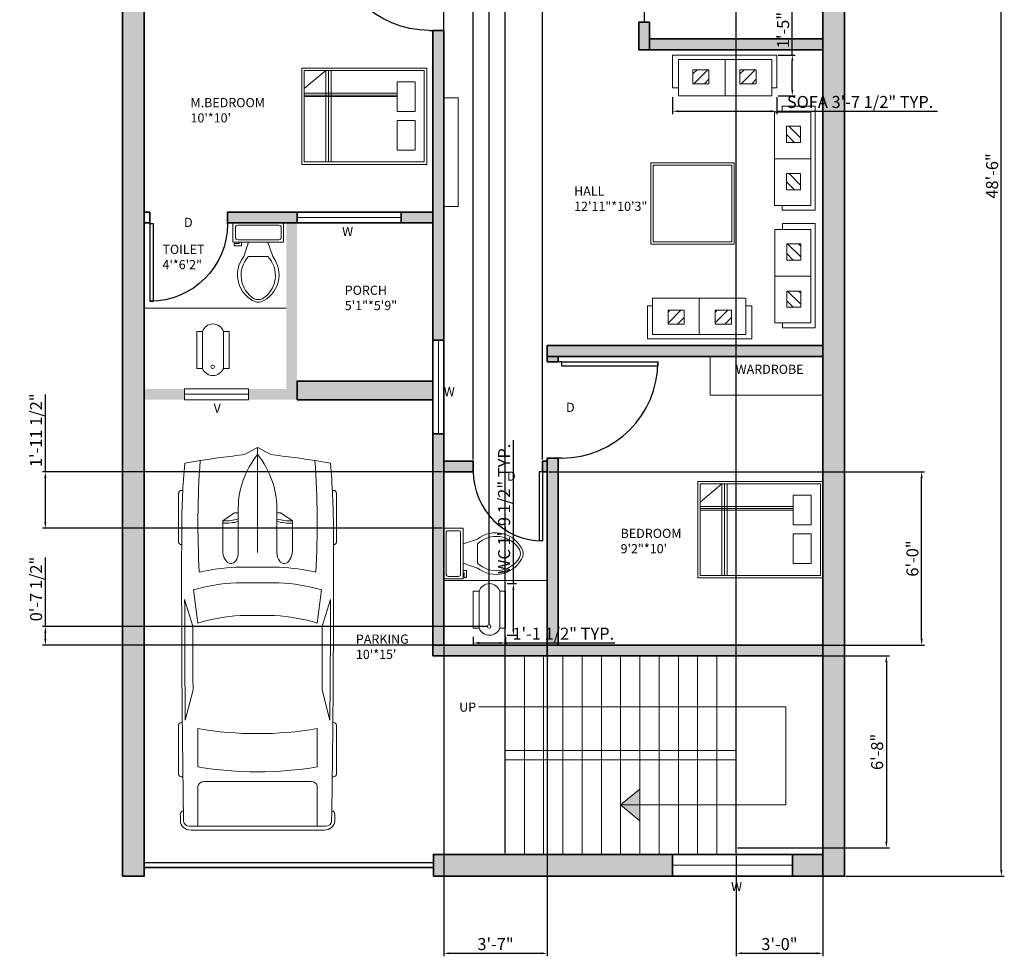
# Model space of a CAD drawing. Units: inches. Extents: x 2318 to 2727, y 1180 to 1889.
# Tile 1 of 2: x 2318 to 2727, y 1180 to 1570. Entities that reach past the tile are written whole.
import ezdxf

# ---------------------------------------------------------------- set-up
doc = ezdxf.new("R2010")
doc.units = ezdxf.units.IN
for name, color, linetype, lineweight in [('A-ANNO-DIMS', 2, 'Continuous', 18), ('A-ANNO-SYMB', 7, 'Continuous', 18), ('A-ANNO-TEXT', 7, 'Continuous', 18), ('A-AREA-IDEN', 7, 'Continuous', 18), ('A-FLOR', 7, 'Continuous', 18), ('A-FLOR-CASE', 52, 'Continuous', 20), ('A-FLOR-FIXT', 9, 'Continuous', 18), ('A-FLOR-STRS', 7, 'Continuous', 18), ('A-FURN', 52, 'Continuous', 18), ('A-WALL-PATT', 192, 'Continuous', 13), ('BED', 52, 'Continuous', 18), ('CAR', 90, 'Continuous', 13), ('DOOR', 20, 'Continuous', 25), ('WALL', 192, 'Continuous', 35), ('WIND', 130, 'Continuous', 20)]:
    doc.layers.add(name, color=color, linetype=linetype, lineweight=lineweight)
doc.styles.get("Standard").update_dxf_attribs({"font": 'arial.ttf'})
doc.dimstyles.new('ISO-25', dxfattribs={"dimtxt": 5, "dimasz": 2.5, "dimexe": 1.25, "dimexo": 0.625, "dimtad": 1, "dimdec": 0, "dimlunit": 4, "dimtxsty": 'Standard', "dimcen": 2.5, "dimadec": 0, "dimazin": 0, "dimtfac": 1, "dimtdec": 0, "dimtmove": 0, "dimatfit": 3, "dimfxl": 1, "dimarcsym": 0})

# ---------------------------------------------------------------- blocks, each defined once
blk = doc.blocks.new('*U6')
for p, q in [((46.55, 38.89), (22.35, 38.89)), ((136.7, 38.89), (160.9, 38.89)), ((21.1, 37.41), (21.1, 36.83)), ((47.8, 37.39), (47.8, 37.41)), ((87.99, 31.87), (74.76, 35.92)), ((134.31, 35.6), (119.29, 31.78)), ((135.45, 37.07), (135.45, 37.41)), ((162.15, 37.41), (162.15, 36.77)), ((70.03, 31.54), (86.41, 29.35)), ((138.42, 29.35), (157.25, 29.35)), ((186.47, 29.35), (167.01, 29.35)), ((186.47, -33.5), (186.47, 33.5)), ((188.4, -32.76), (188.4, 32.76)), ((164.52, 26.39), (164.52, -26.39)), ((32.27, 11.63), (36.13, 17.17)), ((36.13, 17.17), (50.94, 17.17)), ((32.12, 9.51), (32.12, 11.15)), ((58.92, -10.77), (58.92, 10.77)), ((66.55, -10.53), (66.55, 10.53)), ((186.47, -10.53), (186.47, 10.53)), ((3.27, 6.13), (0.1, 0.41)), ((29.77, 9.51), (51.68, 9.51)), ((82.74, 8.5), (82.74, -8.5)), ((0, 0), (51.68, 0)), ((0.1, -0.41), (3.27, -6.13)), ((29.77, -9.51), (51.68, -9.51)), ((32.12, -9.51), (32.12, -11.15)), ((32.27, -11.63), (36.13, -17.17)), ((36.13, -17.17), (50.94, -17.17)), ((86.41, -29.35), (70.03, -31.54)), ((87.99, -31.87), (74.76, -35.92)), ((134.31, -35.6), (119.29, -31.78)), ((157.25, -29.35), (138.42, -29.35)), ((167.01, -29.35), (186.47, -29.35)), ((21.1, -37.41), (21.1, -36.83)), ((47.8, -37.39), (47.8, -37.41)), ((135.45, -37.07), (135.45, -37.41)), ((162.15, -37.41), (162.15, -36.77)), ((46.55, -38.89), (22.35, -38.89)), ((136.7, -38.89), (160.9, -38.89))]:
    blk.add_line(p, q)
for centre, major_axis, ratio, start_param, end_param in [((22.35, 37.41), (0, -1.48), 0.842304, 3.141593, 4.712389), ((46.55, 37.41), (0, 1.48), 0.842304, -1.570796, 0), ((136.7, 37.41), (0, -1.48), 0.842304, 3.141593, 4.712389), ((160.9, 37.41), (0, 1.48), 0.842304, -1.570796, 0), ((266.03, -27.52), (0, 313.31), 0.842304, 1.367076, 1.39176), ((41.19, -490.86), (0, 528.23), 0.842304, 0.00281, 0.075598), ((64.48, -10555.62), (0, 10593.03), 0.842304, -0.013397, 0.002797), ((64.48, -10555.62), (0, -10591.55), 0.842304, 3.133765, 3.140441), ((180.63, 35.84), (0, 2.22), 0.842304, -0.013017, 1.249894), ((64.48, -10556.36), (0, 10595.31), 0.842304, -0.013397, -0.013017), ((183.98, 33.5), (0, -2.96), 0.842304, 1.570796, 3.128196), ((183.98, 32.76), (0, -5.25), 0.842304, 1.570796, 3.128196), ((37.47, -593.96), (0, -623.33), 0.842304, 3.096046, 3.200911), ((135.29, 5.39), (0, 81.77), 0.842304, 1.245306, 1.50788), ((149.6, 2.8), (0, -79.58), 0.842304, 4.372215, 4.640744), ((95.79, -3666.35), (0, -3698.24), 0.842304, 3.134049, 3.144098), ((17.08, 0), (0, 147.02), 0.842304, 4.511394, 4.913384), ((35.91, 0), (0, 147.02), 0.842304, 4.511394, 4.913384), ((167.01, 26.39), (0, 2.96), 0.842304, 0, 1.570796), ((259.18, -27.52), (0, -305.3), 0.842304, 4.528606, 4.561838), ((134.4, 5.39), (0, -89.78), 0.842304, 4.449482, 4.652344), ((-204.49, 52.4), (0, -250.96), 0.842304, 1.385369, 1.434372), ((13.04, 17.01), (0, 27.42), 0.842304, 4.435146, 4.718221), ((14.2, 17.01), (0, 27.42), 0.842304, 4.435146, 4.718221), ((50.79, 13.34), (6.34, -0.36), 0.603834, -1.395552, 1.581315), ((32.75, 11.15), (0, 0.74), 0.842304, 0.879714, 1.570796), ((29.77, -46.66), (0, 56.17), 0.842304, 0, 0.590319), ((0.62, 0), (0, -0.74), 0.842304, 4.131459, 5.293319), ((29.77, 46.66), (0, 56.17), 0.842304, 2.551274, 3.141593), ((-204.49, -52.4), (0, 250.96), 0.842304, -1.434372, -1.385369), ((13.04, -17.01), (0, -27.42), 0.842304, 1.564964, 1.848039), ((14.2, -17.01), (0, -27.42), 0.842304, 1.564964, 1.848039), ((149.6, -2.8), (0, -79.58), 0.842304, -1.499151, -1.230623), ((32.75, -11.15), (0, -0.74), 0.842304, 4.712389, 5.403472), ((134.4, -5.39), (0, -89.78), 0.842304, -1.510751, -1.307889), ((135.29, -5.39), (0, -81.77), 0.842304, -1.50788, -1.245306), ((259.18, 27.52), (0, 305.3), 0.842304, 1.721348, 1.754579), ((266.03, 27.52), (0, 313.31), 0.842304, 1.749832, 1.774517), ((37.47, 593.96), (0, -623.33), 0.842304, -0.059319, 0.045547), ((167.01, -26.39), (0, -2.96), 0.842304, 4.712389, 6.283185), ((95.79, 3666.35), (0, -3698.24), 0.842304, -0.002505, 0.007544), ((183.98, -33.5), (0, 2.96), 0.842304, 3.15499, 4.712389), ((183.98, -32.76), (0, -5.25), 0.842304, 0.013397, 1.570796), ((41.19, 490.86), (0, -528.23), 0.842304, -0.075598, -0.00281), ((22.35, -37.41), (0, 1.48), 0.842304, 1.570796, 3.141593), ((64.48, 10555.62), (0, 10593.03), 0.842304, 3.138796, 3.15499), ((46.55, -37.41), (0, -1.48), 0.842304, 0, 1.570796), ((64.48, 10555.62), (0, -10591.55), 0.842304, 0.001152, 0.007828), ((136.7, -37.41), (0, -1.48), 0.842304, -1.570796, 0), ((160.9, -37.41), (0, 1.48), 0.842304, 3.141593, 4.712389), ((180.63, -35.84), (0, -2.22), 0.842304, -1.249894, 0.013017), ((64.48, 10556.36), (0, 10595.31), 0.842304, 3.15461, 3.15499)]:
    blk.add_ellipse(centre, major_axis=major_axis, ratio=ratio, start_param=start_param, end_param=end_param)
at = {"extrusion": (0, 0, -1)}
blk.add_ellipse((50.79, -13.34), major_axis=(6.34, 0.36), ratio=0.603834, start_param=-1.395552, end_param=1.581315, dxfattribs=at)
blk = doc.blocks.new('*U2')
for p, q in [((0, 0), (0, -6)), ((40, 0), (40, -6))]:
    blk.add_line(p, q)
blk.add_lwpolyline([(0, 0), (0, 40), (1.75, 40), (1.75, 0)], close=True)
blk.add_arc((0, 0), 40, 0, 90)
blk = doc.blocks.new('*U4')
for p, q in [((9.5, -6), (9.5, -2)), ((-8, -8.5), (-8, -8)), ((-7, -8), (-7, -9.5)), ((-4, -8), (-6, -14)), ((4, -8), (6, -14)), ((-10, -8.5), (-8, -8.5)), ((-10, -9.5), (-10, -8.5)), ((-7, -9.5), (-10, -9.5)), ((4, -14), (-4, -14))]:
    blk.add_line(p, q)
blk.add_lwpolyline([(10.5, -8), (10.5, 0), (-10.5, 0), (-10.5, -8)], close=True)
for points in [[(-9.5, -2), (-9.5, -6)], [(8.5, -1), (-8.5, -1)], [(-8.5, -7), (8.5, -7)]]:
    blk.add_lwpolyline(points)
for centre, radius, start, end in [((-8.62, -1.88), 0.884, 81.8699, 188.1301), ((8.62, -1.88), 0.884, 351.8699, 98.1301), ((-8.62, -6.12), 0.884, 171.8699, 278.1301), ((8.62, -6.12), 0.884, 261.8699, 8.1301), ((3.52, -21.58), 12.17, 141.4691, 247.9714), ((4.2, -21.82), 11.33, 136.3677, 238.9468), ((-3.52, -21.58), 12.17, 292.0284, 38.5307), ((-4.2, -21.82), 11.33, 301.053, 43.6321), ((0, -27.88), 4, 245.7318, 294.2682), ((0, -29), 4, 254.8605, 285.1395)]:
    blk.add_arc(centre, radius, start, end)
blk = doc.blocks.new('*D9')
at = {"layer": 'A-ANNO-DIMS', "color": 0, "lineweight": -2, "transparency": 16777216}
for p, q in [((2616.06, 1305.12), (2679.12, 1305.12)), ((2677.87, 1302.62), (2677.87, 1227.86)), ((2616.06, 1225.36), (2679.12, 1225.36))]:
    blk.add_line(p, q, dxfattribs=at)
at = {"layer": 'A-ANNO-DIMS', "color": 0, "transparency": 16777216}
for points in [[(2677.45, 1302.62), (2678.29, 1302.62), (2677.87, 1305.12)], [(2677.45, 1227.86), (2678.29, 1227.86), (2677.87, 1225.36)]]:
    blk.add_solid(points, dxfattribs=at)
at = {"layer": 'Defpoints', "color": 0, "transparency": 16777216}
for p in [(2615.43, 1305.12), (2615.43, 1225.36), (2677.87, 1225.36)]:
    blk.add_point(p, dxfattribs=at)
at = {"layer": 'A-ANNO-DIMS', "color": 0, "transparency": 16777216, "insert": (2674.69, 1265.24), "char_height": 5, "attachment_point": 5, "rotation": 90}
blk.add_mtext('6\'-8"', dxfattribs=at)
blk = doc.blocks.new('*D10')
at = {"layer": 'A-ANNO-DIMS', "color": 0, "lineweight": -2, "transparency": 16777216}
for p, q in [((2661.06, 1795.62), (2726.9, 1795.62)), ((2725.65, 1216.12), (2725.65, 1793.12)), ((2661.06, 1213.62), (2726.9, 1213.62))]:
    blk.add_line(p, q, dxfattribs=at)
at = {"layer": 'A-ANNO-DIMS', "color": 0, "transparency": 16777216}
for points in [[(2725.23, 1793.12), (2726.06, 1793.12), (2725.65, 1795.62)], [(2725.23, 1216.12), (2726.06, 1216.12), (2725.65, 1213.62)]]:
    blk.add_solid(points, dxfattribs=at)
at = {"layer": 'Defpoints', "color": 0, "transparency": 16777216}
for p in [(2660.43, 1795.62), (2725.65, 1795.62), (2660.43, 1213.62)]:
    blk.add_point(p, dxfattribs=at)
at = {"layer": 'A-ANNO-DIMS', "color": 0, "transparency": 16777216, "insert": (2722.47, 1504.62), "char_height": 5, "attachment_point": 5, "rotation": 90}
blk.add_mtext('48\'-6"', dxfattribs=at)
blk = doc.blocks.new('BED-DOUBLE')
for p, q in [((1, 31.46), (10.01, 39.03)), ((10.01, 39.03), (10.01, 1)), ((11.11, 39.03), (11.11, 1)), ((12.24, 39.03), (12.24, 1)), ((39.72, 29.6), (1, 29.6)), ((1, 28.8), (39.72, 28.8)), ((39.72, 28.17), (1, 28.17))]:
    blk.add_line(p, q)
for points in [[(51.96, 40.03), (0, 40.03), (0, 0), (51.96, 0)], [(50.96, 39.03), (1, 39.03), (1, 1), (50.96, 1)], [(47.18, 34.34), (39.72, 34.34), (39.72, 22.01), (47.18, 22.01)], [(47.18, 18.28), (39.72, 18.28), (39.72, 5.95), (47.18, 5.95)]]:
    blk.add_lwpolyline(points, close=True)
blk = doc.blocks.new('WC-SQUAT')
for points in [[(0, 2.9), (2.39, 2.9), (2.39, 18.34), (0, 18.34)], [(11.06, 2.9), (13.46, 2.9), (13.46, 18.34), (11.06, 18.34)]]:
    blk.add_lwpolyline(points, close=True)
for points in [[(2.39, 18.28), (2.39, 2.9)], [(11.06, 2.9), (11.06, 18.28)]]:
    blk.add_lwpolyline(points)
blk.add_circle((6.6, 3.6), 0.726)
for centre, radius, start, end in [((6.73, 16.89), 4.55, 17.8162, 162.1838), ((6.73, 4.69), 4.69, 202.5147, 337.4853)]:
    blk.add_arc(centre, radius, start, end)
blk = doc.blocks.new('SOFA-TWO-SEAT')
h = blk.add_hatch()
h.set_pattern_fill('ANSI31', color=256)
h.set_pattern_definition([(45, (-2589.011, -1538.005), (-2.245064, 2.245064), [])])
h.paths.add_polyline_path([(15.14, 10.8), (8.38, 10.8), (8.38, 4.98), (15.14, 4.98)])
h = blk.add_hatch()
h.set_pattern_fill('ANSI31', color=256)
h.set_pattern_definition([(45, (-2569.365, -1538.005), (-2.245064, 2.245064), [])])
h.paths.add_polyline_path([(34.79, 10.8), (28.03, 10.8), (28.03, 4.98), (34.79, 4.98)])
for p, q in [((0, 3.19), (0, 16.86)), ((0, 16.86), (43.28, 16.86)), ((43.28, 16.86), (43.28, 3.19)), ((21.85, 0), (21.85, 15.05)), ((2.44, 3.19), (0, 3.19)), ((43.28, 3.19), (41.27, 3.19))]:
    blk.add_line(p, q)
for points in [[(2.44, 0), (41.27, 0), (41.27, 15.05), (2.44, 15.05)], [(8.38, 4.98), (15.14, 4.98), (15.14, 10.8), (8.38, 10.8)], [(28.03, 4.98), (34.79, 4.98), (34.79, 10.8), (28.03, 10.8)]]:
    blk.add_lwpolyline(points, close=True)
blk = doc.blocks.new('*D16')
at = {"layer": 'A-ANNO-DIMS', "color": 0, "lineweight": -2, "transparency": 16777216}
for p, q in [((2589.01, 1537.38), (2589.01, 1530.26)), ((2632.29, 1537.38), (2632.29, 1530.26)), ((2591.51, 1531.51), (2629.79, 1531.51)), ((2632.29, 1531.51), (2699.11, 1531.51))]:
    blk.add_line(p, q, dxfattribs=at)
at = {"layer": 'A-ANNO-DIMS', "color": 0, "transparency": 16777216}
for points in [[(2591.51, 1531.93), (2591.51, 1531.1), (2589.01, 1531.51)], [(2629.79, 1531.93), (2629.79, 1531.1), (2632.29, 1531.51)]]:
    blk.add_solid(points, dxfattribs=at)
at = {"layer": 'Defpoints', "color": 0, "transparency": 16777216}
for p in [(2589.01, 1538), (2632.29, 1538), (2632.29, 1531.51)]:
    blk.add_point(p, dxfattribs=at)
at = {"layer": 'A-ANNO-DIMS', "color": 0, "transparency": 16777216, "insert": (2666.95, 1534.73), "char_height": 5, "attachment_point": 5}
blk.add_mtext('SOFA 3\'-7 1/2" TYP.', dxfattribs=at)
blk = doc.blocks.new('*D17')
at = {"layer": 'A-ANNO-DIMS', "color": 0, "lineweight": -2, "transparency": 16777216}
for p, q in [((2638.78, 1554.87), (2638.78, 1588.62)), ((2632.92, 1554.87), (2640.03, 1554.87)), ((2638.78, 1540.5), (2638.78, 1552.37)), ((2632.92, 1538), (2640.03, 1538))]:
    blk.add_line(p, q, dxfattribs=at)
at = {"layer": 'A-ANNO-DIMS', "color": 0, "transparency": 16777216}
for points in [[(2638.37, 1552.37), (2639.2, 1552.37), (2638.78, 1554.87)], [(2638.37, 1540.5), (2639.2, 1540.5), (2638.78, 1538)]]:
    blk.add_solid(points, dxfattribs=at)
at = {"layer": 'Defpoints', "color": 0, "transparency": 16777216}
for p in [(2632.29, 1554.87), (2638.78, 1554.87), (2632.29, 1538)]:
    blk.add_point(p, dxfattribs=at)
at = {"layer": 'A-ANNO-DIMS', "color": 0, "transparency": 16777216, "insert": (2635.61, 1572.99), "char_height": 5, "attachment_point": 5, "rotation": 90}
blk.add_mtext('1\'-5" TYP.', dxfattribs=at)
blk = doc.blocks.new('*D20')
at = {"layer": 'A-ANNO-DIMS', "color": 0, "lineweight": -2, "transparency": 16777216}
for p, q in [((2522.86, 1335.18), (2522.86, 1394.84)), ((2520.26, 1335.18), (2524.11, 1335.18)), ((2522.86, 1316.23), (2522.86, 1332.68)), ((2520.26, 1313.73), (2524.11, 1313.73))]:
    blk.add_line(p, q, dxfattribs=at)
at = {"layer": 'A-ANNO-DIMS', "color": 0, "transparency": 16777216}
for points in [[(2522.44, 1332.68), (2523.27, 1332.68), (2522.86, 1335.18)], [(2522.44, 1316.23), (2523.27, 1316.23), (2522.86, 1313.73)]]:
    blk.add_solid(points, dxfattribs=at)
at = {"layer": 'Defpoints', "color": 0, "transparency": 16777216}
for p in [(2519.64, 1335.18), (2522.86, 1335.18), (2519.64, 1313.73)]:
    blk.add_point(p, dxfattribs=at)
at = {"layer": 'A-ANNO-DIMS', "color": 0, "transparency": 16777216, "insert": (2519.65, 1366.26), "char_height": 5, "attachment_point": 5, "rotation": 90}
blk.add_mtext('WC 1\'-9 1/2" TYP.', dxfattribs=at)
blk = doc.blocks.new('*D21')
at = {"layer": 'A-ANNO-DIMS', "color": 0, "lineweight": -2, "transparency": 16777216}
for p, q in [((2506.18, 1313.11), (2506.18, 1309.26)), ((2508.68, 1310.51), (2517.14, 1310.51)), ((2519.64, 1313.11), (2519.64, 1309.26)), ((2519.64, 1310.51), (2565.05, 1310.51))]:
    blk.add_line(p, q, dxfattribs=at)
at = {"layer": 'A-ANNO-DIMS', "color": 0, "transparency": 16777216}
for points in [[(2508.68, 1310.93), (2508.68, 1310.1), (2506.18, 1310.51)], [(2517.14, 1310.93), (2517.14, 1310.1), (2519.64, 1310.51)]]:
    blk.add_solid(points, dxfattribs=at)
at = {"layer": 'Defpoints', "color": 0, "transparency": 16777216}
for p in [(2506.18, 1313.73), (2519.64, 1313.73), (2519.64, 1310.51)]:
    blk.add_point(p, dxfattribs=at)
at = {"layer": 'A-ANNO-DIMS', "color": 0, "transparency": 16777216, "insert": (2543.59, 1313.72), "char_height": 5, "attachment_point": 5}
blk.add_mtext('1\'-1 1/2" TYP.', dxfattribs=at)
blk = doc.blocks.new('*D24')
at = {"layer": 'A-ANNO-DIMS', "color": 0, "lineweight": -2, "transparency": 16777216}
for p, q in [((2519.43, 1223.25), (2519.43, 1879.97)), ((2521.93, 1878.72), (2612.93, 1878.72)), ((2615.43, 1223.25), (2615.43, 1879.97))]:
    blk.add_line(p, q, dxfattribs=at)
at = {"layer": 'A-ANNO-DIMS', "color": 0, "transparency": 16777216}
for points in [[(2521.93, 1879.14), (2521.93, 1878.3), (2519.43, 1878.72)], [(2612.93, 1879.14), (2612.93, 1878.3), (2615.43, 1878.72)]]:
    blk.add_solid(points, dxfattribs=at)
at = {"layer": 'Defpoints', "color": 0, "transparency": 16777216}
for p in [(2615.43, 1878.72), (2519.43, 1222.62), (2615.43, 1222.62)]:
    blk.add_point(p, dxfattribs=at)
at = {"layer": 'A-ANNO-DIMS', "color": 0, "transparency": 16777216, "insert": (2567.43, 1881.9), "char_height": 5, "attachment_point": 5}
blk.add_mtext('8\'-0"', dxfattribs=at)
blk = doc.blocks.new('*D25')
at = {"layer": 'A-ANNO-DIMS', "color": 0, "lineweight": -2, "transparency": 16777216}
for p, q in [((2615.43, 1222), (2615.43, 1180.27)), ((2651.43, 1222), (2651.43, 1180.27)), ((2617.93, 1181.52), (2648.93, 1181.52))]:
    blk.add_line(p, q, dxfattribs=at)
at = {"layer": 'A-ANNO-DIMS', "color": 0, "transparency": 16777216}
for points in [[(2617.93, 1181.94), (2617.93, 1181.1), (2615.43, 1181.52)], [(2648.93, 1181.94), (2648.93, 1181.1), (2651.43, 1181.52)]]:
    blk.add_solid(points, dxfattribs=at)
at = {"layer": 'Defpoints', "color": 0, "transparency": 16777216}
for p in [(2615.43, 1222.62), (2651.43, 1222.62), (2651.43, 1181.52)]:
    blk.add_point(p, dxfattribs=at)
at = {"layer": 'A-ANNO-DIMS', "color": 0, "transparency": 16777216, "insert": (2633.43, 1184.7), "char_height": 5, "attachment_point": 5}
blk.add_mtext('3\'-0"', dxfattribs=at)
blk = doc.blocks.new('*D26')
at = {"layer": 'A-ANNO-DIMS', "color": 0, "lineweight": -2, "transparency": 16777216}
for p, q in [((2493.93, 1309), (2493.93, 1180.27)), ((2536.93, 1309), (2536.93, 1180.27)), ((2496.43, 1181.52), (2534.43, 1181.52))]:
    blk.add_line(p, q, dxfattribs=at)
at = {"layer": 'A-ANNO-DIMS', "color": 0, "transparency": 16777216}
for points in [[(2496.43, 1181.94), (2496.43, 1181.1), (2493.93, 1181.52)], [(2534.43, 1181.94), (2534.43, 1181.1), (2536.93, 1181.52)]]:
    blk.add_solid(points, dxfattribs=at)
at = {"layer": 'Defpoints', "color": 0, "transparency": 16777216}
for p in [(2493.93, 1309.62), (2536.93, 1309.62), (2536.93, 1181.52)]:
    blk.add_point(p, dxfattribs=at)
at = {"layer": 'A-ANNO-DIMS', "color": 0, "transparency": 16777216, "insert": (2515.43, 1184.7), "char_height": 5, "attachment_point": 5}
blk.add_mtext('3\'-7"', dxfattribs=at)
blk = doc.blocks.new('*D27')
at = {"layer": 'A-ANNO-DIMS', "color": 0, "lineweight": -2, "transparency": 16777216}
for p, q in [((2537.56, 1381.62), (2693.78, 1381.62)), ((2692.53, 1312.12), (2692.53, 1379.12)), ((2537.56, 1309.62), (2693.78, 1309.62))]:
    blk.add_line(p, q, dxfattribs=at)
at = {"layer": 'A-ANNO-DIMS', "color": 0, "transparency": 16777216}
for points in [[(2692.12, 1379.12), (2692.95, 1379.12), (2692.53, 1381.62)], [(2692.12, 1312.12), (2692.95, 1312.12), (2692.53, 1309.62)]]:
    blk.add_solid(points, dxfattribs=at)
at = {"layer": 'Defpoints', "color": 0, "transparency": 16777216}
for p in [(2536.93, 1381.62), (2692.53, 1381.62), (2536.93, 1309.62)]:
    blk.add_point(p, dxfattribs=at)
at = {"layer": 'A-ANNO-DIMS', "color": 0, "transparency": 16777216, "insert": (2689.36, 1345.62), "char_height": 5, "attachment_point": 5, "rotation": 90}
blk.add_mtext('6\'-0"', dxfattribs=at)
blk = doc.blocks.new('*D28')
at = {"layer": 'A-ANNO-DIMS', "color": 0, "lineweight": -2, "transparency": 16777216}
for p, q in [((2506.2, 1386.75), (2506.2, 1879.97)), ((2508.7, 1878.72), (2532.52, 1878.72)), ((2535.02, 1386.75), (2535.02, 1879.97))]:
    blk.add_line(p, q, dxfattribs=at)
at = {"layer": 'A-ANNO-DIMS', "color": 0, "transparency": 16777216}
for points in [[(2508.7, 1879.14), (2508.7, 1878.3), (2506.2, 1878.72)], [(2532.52, 1879.14), (2532.52, 1878.3), (2535.02, 1878.72)]]:
    blk.add_solid(points, dxfattribs=at)
at = {"layer": 'Defpoints', "color": 0, "transparency": 16777216}
for p in [(2535.02, 1878.72), (2506.2, 1386.12), (2535.02, 1386.12)]:
    blk.add_point(p, dxfattribs=at)
at = {"layer": 'A-ANNO-DIMS', "color": 0, "transparency": 16777216, "insert": (2520.61, 1881.9), "char_height": 5, "attachment_point": 5}
blk.add_mtext('2\'-5"', dxfattribs=at)
blk = doc.blocks.new('*D29')
at = {"layer": 'A-ANNO-DIMS', "color": 0, "lineweight": -2, "transparency": 16777216}
for p, q in [((2493.93, 1386.75), (2493.93, 1879.97)), ((2496.43, 1878.72), (2503.7, 1878.72)), ((2506.2, 1386.75), (2506.2, 1879.97)), ((2506.2, 1878.72), (2534.42, 1878.72))]:
    blk.add_line(p, q, dxfattribs=at)
at = {"layer": 'A-ANNO-DIMS', "color": 0, "transparency": 16777216}
for points in [[(2496.43, 1879.14), (2496.43, 1878.3), (2493.93, 1878.72)], [(2503.7, 1879.14), (2503.7, 1878.3), (2506.2, 1878.72)]]:
    blk.add_solid(points, dxfattribs=at)
at = {"layer": 'Defpoints', "color": 0, "transparency": 16777216}
for p in [(2506.2, 1878.72), (2493.93, 1386.12), (2506.2, 1386.12)]:
    blk.add_point(p, dxfattribs=at)
at = {"layer": 'A-ANNO-DIMS', "color": 0, "transparency": 16777216, "insert": (2521.56, 1881.93), "char_height": 5, "attachment_point": 5}
blk.add_mtext('1\'-0 1/2"', dxfattribs=at)
blk = doc.blocks.new('*D30')
at = {"layer": 'A-ANNO-DIMS', "color": 0, "lineweight": -2, "transparency": 16777216}
for p, q in [((2493.93, 1310.25), (2493.93, 1879.97)), ((2496.43, 1878.72), (2510.28, 1878.72)), ((2512.78, 1317.96), (2512.78, 1879.97))]:
    blk.add_line(p, q, dxfattribs=at)
at = {"layer": 'A-ANNO-DIMS', "color": 0, "transparency": 16777216}
for points in [[(2496.43, 1879.14), (2496.43, 1878.3), (2493.93, 1878.72)], [(2510.28, 1879.14), (2510.28, 1878.3), (2512.78, 1878.72)]]:
    blk.add_solid(points, dxfattribs=at)
at = {"layer": 'Defpoints', "color": 0, "transparency": 16777216}
for p in [(2512.78, 1878.72), (2512.78, 1317.33), (2493.93, 1309.62)]:
    blk.add_point(p, dxfattribs=at)
at = {"layer": 'A-ANNO-DIMS', "color": 0, "transparency": 16777216, "insert": (2503.36, 1881.86), "char_height": 5, "attachment_point": 5}
blk.add_mtext('1\'-7"', dxfattribs=at)
blk = doc.blocks.new('*D31')
at = {"layer": 'A-ANNO-DIMS', "color": 0, "lineweight": -2, "transparency": 16777216}
for p, q in [((2328.33, 1317.33), (2328.33, 1346.02)), ((2512.16, 1317.33), (2327.08, 1317.33)), ((2328.33, 1312.12), (2328.33, 1314.83)), ((2493.31, 1309.62), (2327.08, 1309.62))]:
    blk.add_line(p, q, dxfattribs=at)
at = {"layer": 'A-ANNO-DIMS', "color": 0, "transparency": 16777216}
for points in [[(2327.92, 1314.83), (2328.75, 1314.83), (2328.33, 1317.33)], [(2327.92, 1312.12), (2328.75, 1312.12), (2328.33, 1309.62)]]:
    blk.add_solid(points, dxfattribs=at)
at = {"layer": 'Defpoints', "color": 0, "transparency": 16777216}
for p in [(2328.33, 1317.33), (2512.78, 1317.33), (2493.93, 1309.62)]:
    blk.add_point(p, dxfattribs=at)
at = {"layer": 'A-ANNO-DIMS', "color": 0, "transparency": 16777216, "insert": (2325.12, 1332.93), "char_height": 5, "attachment_point": 5, "rotation": 90}
blk.add_mtext('0\'-7 1/2"', dxfattribs=at)
blk = doc.blocks.new('*D32')
at = {"layer": 'A-ANNO-DIMS', "color": 0, "lineweight": -2, "transparency": 16777216}
for p, q in [((2328.33, 1381.62), (2328.33, 1413.73)), ((2493.31, 1381.62), (2327.08, 1381.62)), ((2328.33, 1360.67), (2328.33, 1379.12)), ((2493.31, 1358.17), (2327.08, 1358.17))]:
    blk.add_line(p, q, dxfattribs=at)
at = {"layer": 'A-ANNO-DIMS', "color": 0, "transparency": 16777216}
for points in [[(2327.92, 1379.12), (2328.75, 1379.12), (2328.33, 1381.62)], [(2327.92, 1360.67), (2328.75, 1360.67), (2328.33, 1358.17)]]:
    blk.add_solid(points, dxfattribs=at)
at = {"layer": 'Defpoints', "color": 0, "transparency": 16777216}
for p in [(2328.33, 1381.62), (2493.93, 1381.62), (2493.93, 1358.17)]:
    blk.add_point(p, dxfattribs=at)
at = {"layer": 'A-ANNO-DIMS', "color": 0, "transparency": 16777216, "insert": (2325.12, 1398.92), "char_height": 5, "attachment_point": 5, "rotation": 90}
blk.add_mtext('1\'-11 1/2"', dxfattribs=at)

msp = doc.modelspace()

# ---------------------------------------------------------------- hatches: boundary and pattern name
at = {"layer": 'A-ANNO-SYMB'}
h = msp.add_hatch(color=256, dxfattribs=at)
h.dxf.hatch_style = 1
h.paths.add_polyline_path([(2575.43, 1249.74), (2567.43, 1243.17), (2575.43, 1243.17)])
h.paths.add_polyline_path([(2575.43, 1243.17), (2567.43, 1243.17), (2575.43, 1236.61)])
at = {"layer": 'A-WALL-PATT'}
h = msp.add_hatch(color=256, dxfattribs=at)
h.dxf.hatch_style = 1
h.paths.add_polyline_path([(2651.43, 1795.62), (2360.43, 1795.62), (2360.43, 1786.62), (2369.43, 1786.62), (2651.43, 1786.62)])
h.paths.add_polyline_path([(2481.93, 1786.62), (2477.43, 1786.62), (2477.43, 1778.41), (2481.93, 1778.41)])
h.paths.add_polyline_path([(2481.93, 1750.36), (2477.43, 1750.36), (2477.43, 1738.62), (2481.93, 1738.62)])
h.paths.add_polyline_path([(2369.43, 1786.62), (2360.43, 1786.62), (2360.43, 1213.62), (2369.43, 1213.62)])
h.paths.add_polyline_path([(2660.43, 1795.62), (2651.43, 1795.62), (2651.43, 1786.62), (2651.43, 1213.62), (2660.43, 1213.62)])
h.paths.add_polyline_path([(2496.41, 1614.12), (2369.43, 1614.12), (2369.43, 1609.62), (2496.41, 1609.62)])
h.paths.add_polyline_path([(2651.43, 1614.12), (2570.03, 1614.12), (2570.03, 1609.62), (2651.43, 1609.62)])
h.paths.add_polyline_path([(2579.43, 1609.62), (2574.93, 1609.62), (2574.93, 1602.98), (2579.43, 1602.98)])
h.paths.add_polyline_path([(2579.43, 1568.54), (2574.93, 1568.54), (2574.93, 1557.12), (2579.43, 1557.12)])
h.paths.add_polyline_path([(2651.43, 1561.62), (2579.43, 1561.62), (2579.43, 1557.12), (2651.43, 1557.12)])
h.paths.add_polyline_path([(2493.93, 1565.11), (2489.43, 1565.11), (2489.43, 1436.36), (2493.93, 1436.36)])
h.paths.add_polyline_path([(2489.43, 1419.4), (2432.93, 1419.4), (2432.93, 1411.62), (2489.43, 1411.62)])
h.paths.add_polyline_path([(2493.93, 1397.39), (2489.43, 1397.39), (2489.43, 1309.62), (2493.93, 1309.62)])
h.paths.add_polyline_path([(2506.2, 1386.12), (2493.93, 1386.12), (2493.93, 1381.62), (2506.2, 1381.62)])
h.paths.add_polyline_path([(2651.43, 1434.12), (2536.93, 1434.12), (2536.93, 1429.62), (2651.43, 1429.62)])
h.paths.add_polyline_path([(2541.43, 1429.62), (2536.93, 1429.62), (2536.93, 1427.36), (2541.43, 1427.36)])
h.paths.add_polyline_path([(2541.43, 1387.36), (2536.93, 1387.36), (2536.93, 1309.62), (2541.43, 1309.62)])
h.paths.add_polyline_path([(2536.93, 1386.12), (2535.02, 1386.12), (2535.02, 1381.8), (2535.02, 1381.62), (2536.93, 1381.62)])
h.paths.add_polyline_path([(2536.93, 1309.62), (2489.43, 1309.62), (2489.43, 1305.12), (2536.93, 1305.12)])
h.paths.add_polyline_path([(2651.43, 1309.62), (2536.93, 1309.62), (2536.93, 1305.12), (2651.43, 1305.12)])
h.paths.add_polyline_path([(2651.43, 1222.62), (2638.9, 1222.62), (2638.9, 1213.62), (2651.43, 1213.62)])
h.paths.add_polyline_path([(2588.94, 1222.62), (2489.59, 1222.62), (2489.59, 1213.62), (2588.94, 1213.62)])
h = msp.add_hatch(color=256, dxfattribs=at)
h.dxf.hatch_style = 1
h.paths.add_polyline_path([(2481.93, 1738.62), (2477.43, 1738.62), (2404.9, 1738.62), (2404.9, 1734.12), (2481.93, 1734.12)])
h.paths.add_polyline_path([(2537.33, 1738.62), (2529.86, 1738.62), (2529.86, 1734.12), (2530.43, 1734.12), (2530.43, 1614.12), (2534.93, 1614.12), (2534.93, 1734.12), (2537.33, 1734.12)])
h.paths.add_polyline_path([(2599, 1738.62), (2588.85, 1738.62), (2588.85, 1734.12), (2599, 1734.12)])
h.paths.add_polyline_path([(2651.43, 1738.62), (2645.81, 1738.62), (2645.81, 1734.12), (2651.43, 1734.12)])
h.paths.add_polyline_path([(2534.93, 1614.12), (2530.43, 1614.12), (2530.3, 1614.12), (2530.3, 1609.62), (2534.93, 1609.62)])
h.paths.add_polyline_path([(2493.93, 1609.62), (2489.43, 1609.62), (2489.43, 1605.11), (2493.93, 1605.11)])
h.paths.add_polyline_path([(2386.22, 1416.12), (2369.43, 1416.12), (2369.43, 1411.62), (2386.22, 1411.62)])
h.paths.add_polyline_path([(2432.93, 1416.12), (2432.93, 1485.12), (2428.43, 1485.12), (2428.43, 1416.12), (2412.83, 1416.12), (2412.83, 1411.62), (2428.43, 1411.62), (2432.93, 1411.62)])
h = msp.add_hatch(color=256, dxfattribs=at)
h.dxf.hatch_style = 1
h.paths.add_polyline_path([(2489.43, 1489.62), (2476.24, 1489.62), (2476.24, 1485.12), (2489.43, 1485.12)])
h.paths.add_polyline_path([(2432.93, 1489.62), (2404.06, 1489.62), (2404.06, 1485.12), (2432.93, 1485.12)])

# ---------------------------------------------------------------- linework, layer by layer
at = {"layer": 'A-ANNO-SYMB'}
for p, q in [((2508.53, 1283.98), (2636.15, 1283.98)), ((2636.15, 1283.98), (2636.15, 1243.17)), ((2567.43, 1243.17), (2575.43, 1249.74)), ((2636.15, 1243.17), (2567.43, 1243.17)), ((2567.43, 1243.17), (2575.43, 1236.61))]:
    msp.add_line(p, q, dxfattribs=at)
at = {"layer": 'A-FLOR'}
for p, q in [((2369.43, 1449.69), (2428.43, 1449.69)), ((2493.93, 1336.53), (2536.93, 1336.53))]:
    msp.add_line(p, q, dxfattribs=at)
at = {"layer": 'A-FLOR-CASE'}
for points in [[(2493.93, 1491.99), (2499.84, 1491.99), (2499.84, 1537.16), (2493.93, 1537.16)], [(2651.43, 1429.62), (2604.68, 1429.62), (2604.68, 1413.49), (2651.43, 1413.49)]]:
    msp.add_lwpolyline(points, close=True, dxfattribs=at)
at = {"layer": 'A-FLOR-STRS'}
for p, q in [((2519.43, 1305.12), (2519.43, 1222.62)), ((2527.43, 1305.12), (2527.43, 1222.62)), ((2535.43, 1305.12), (2535.43, 1222.62)), ((2543.43, 1305.12), (2543.43, 1222.62)), ((2543.43, 1305.12), (2543.43, 1222.62)), ((2551.43, 1305.12), (2551.43, 1222.62)), ((2559.43, 1305.12), (2559.43, 1222.62)), ((2567.43, 1305.12), (2567.43, 1222.62)), ((2575.43, 1305.12), (2575.43, 1222.62)), ((2583.43, 1305.12), (2583.43, 1222.62)), ((2591.43, 1305.12), (2591.43, 1222.62)), ((2599.43, 1305.12), (2599.43, 1222.62)), ((2607.43, 1305.12), (2607.43, 1222.62)), ((2651.43, 1305.12), (2615.43, 1305.12)), ((2615.43, 1305.12), (2615.43, 1222.62)), ((2615.43, 1265.87), (2519.1, 1265.87)), ((2615.43, 1261.87), (2519.1, 1261.87))]:
    msp.add_line(p, q, dxfattribs=at)
at = {"layer": 'A-FURN'}
for points in [[(2614.67, 1476.3), (2580.01, 1476.3), (2580.01, 1510.09), (2614.67, 1510.09)], [(2613.67, 1477.3), (2581.01, 1477.3), (2581.01, 1509.09), (2613.67, 1509.09)]]:
    msp.add_lwpolyline(points, close=True, dxfattribs=at)
at = {"layer": 'DOOR'}
for p, q in [((2577.18, 1602.98), (2577.18, 1568.54)), ((2489.37, 1217.14), (2369.22, 1217.14)), ((2489.59, 1219.12), (2369.43, 1219.12))]:
    msp.add_line(p, q, dxfattribs=at)
msp.add_lwpolyline([(2369.43, 1217.14), (2489.59, 1217.14), (2489.59, 1219.12), (2369.43, 1219.12)], close=True, dxfattribs=at)
at = {"layer": 'WALL'}
for p, q in [((2360.43, 1213.62), (2360.43, 1795.62)), ((2660.43, 1795.62), (2660.43, 1213.62)), ((2651.43, 1609.62), (2651.43, 1561.62)), ((2574.93, 1557.12), (2574.93, 1568.54)), ((2579.43, 1568.54), (2574.93, 1568.54)), ((2579.43, 1561.62), (2579.43, 1568.54)), ((2489.43, 1565.11), (2489.43, 1489.62)), ((2493.93, 1565.11), (2493.93, 1485.12)), ((2651.43, 1561.62), (2579.43, 1561.62)), ((2651.43, 1557.12), (2574.93, 1557.12)), ((2651.43, 1557.12), (2651.43, 1434.12)), ((2371.81, 1489.62), (2369.43, 1489.62)), ((2489.43, 1489.62), (2404.06, 1489.62)), ((2493.93, 1411.62), (2493.93, 1487.37)), ((2369.43, 1485.12), (2371.81, 1485.12)), ((2371.81, 1485.12), (2369.43, 1485.12)), ((2489.43, 1485.12), (2404.06, 1485.12)), ((2404.06, 1485.12), (2417.43, 1485.12)), ((2489.43, 1485.12), (2428.43, 1485.12)), ((2489.43, 1419.4), (2489.43, 1485.12)), ((2651.43, 1434.12), (2536.93, 1434.12)), ((2536.93, 1429.62), (2536.93, 1434.12)), ((2651.43, 1429.62), (2536.93, 1429.62)), ((2536.93, 1427.36), (2536.93, 1429.62)), ((2541.43, 1427.36), (2541.43, 1429.62)), ((2651.43, 1429.62), (2651.43, 1309.62)), ((2432.93, 1419.4), (2432.93, 1416.12)), ((2432.93, 1419.4), (2489.43, 1419.4)), ((2432.93, 1416.12), (2432.93, 1411.62)), ((2432.93, 1411.62), (2489.43, 1411.62)), ((2489.43, 1411.62), (2489.43, 1305.12)), ((2493.93, 1411.62), (2493.93, 1309.62)), ((2536.93, 1305.12), (2536.93, 1387.36)), ((2541.43, 1309.62), (2541.43, 1387.36)), ((2493.93, 1386.12), (2506.2, 1386.12)), ((2535.02, 1386.12), (2536.93, 1386.12)), ((2493.93, 1309.62), (2493.93, 1381.62)), ((2493.93, 1381.62), (2506.2, 1381.62)), ((2493.93, 1309.62), (2541.43, 1309.62)), ((2651.43, 1309.62), (2541.43, 1309.62)), ((2651.43, 1305.12), (2489.43, 1305.12)), ((2369.43, 1222.62), (2369.43, 1213.62)), ((2489.59, 1222.62), (2489.59, 1213.62)), ((2369.43, 1213.62), (2360.43, 1213.62)), ((2660.43, 1213.62), (2489.59, 1213.62))]:
    msp.add_line(p, q, dxfattribs=at)
for points in [[(2369.43, 1213.62), (2360.43, 1213.62), (2360.43, 1795.62), (2660.43, 1795.62), (2660.43, 1213.62), (2489.59, 1213.62)], [(2369.43, 1222.62), (2369.43, 1786.62), (2651.43, 1786.62), (2651.43, 1222.62), (2489.59, 1222.62)], [(2360.43, 1305.89), (2360.43, 1316.22)], [(2369.43, 1316.22), (2369.43, 1305.89)]]:
    msp.add_lwpolyline(points, dxfattribs=at)
for points in [[(2651.43, 1795.62), (2660.43, 1795.62), (2660.43, 1213.62), (2651.43, 1213.62)], [(2360.43, 1213.62), (2369.43, 1213.62), (2369.43, 1786.62), (2360.43, 1786.62)], [(2574.93, 1568.54), (2579.43, 1568.54), (2579.43, 1557.12), (2574.93, 1557.12)], [(2489.43, 1565.11), (2493.93, 1565.11), (2493.93, 1436.36), (2489.43, 1436.36)], [(2651.43, 1557.12), (2579.43, 1557.12), (2579.43, 1561.62), (2651.43, 1561.62)], [(2371.81, 1489.62), (2369.43, 1489.62), (2369.43, 1485.12), (2371.81, 1485.12)], [(2404.06, 1489.62), (2432.93, 1489.62), (2432.93, 1485.12), (2404.06, 1485.12)], [(2476.24, 1489.62), (2489.43, 1489.62), (2489.43, 1485.12), (2476.24, 1485.12)], [(2536.93, 1429.62), (2651.43, 1429.62), (2651.43, 1434.12), (2536.93, 1434.12)], [(2536.93, 1427.36), (2541.43, 1427.36), (2541.43, 1429.62), (2536.93, 1429.62)], [(2432.93, 1411.62), (2489.43, 1411.62), (2489.43, 1419.4), (2432.93, 1419.4)], [(2489.43, 1397.39), (2493.93, 1397.39), (2493.93, 1309.62), (2489.43, 1309.62)], [(2536.93, 1309.62), (2541.43, 1309.62), (2541.43, 1387.36), (2536.93, 1387.36)], [(2506.2, 1381.62), (2493.93, 1381.62), (2493.93, 1386.12), (2506.2, 1386.12)], [(2535.02, 1386.12), (2536.93, 1386.12), (2536.93, 1381.62), (2535.02, 1381.62)], [(2489.43, 1305.12), (2536.93, 1305.12), (2536.93, 1309.62), (2489.43, 1309.62)], [(2536.93, 1305.12), (2651.43, 1305.12), (2651.43, 1309.62), (2536.93, 1309.62)], [(2489.59, 1213.62), (2588.94, 1213.62), (2588.94, 1222.62), (2489.59, 1222.62)], [(2638.9, 1222.62), (2651.43, 1222.62), (2651.43, 1213.62), (2638.9, 1213.62)]]:
    msp.add_lwpolyline(points, close=True, dxfattribs=at)
at = {"layer": 'WIND'}
for p, q in [((2432.93, 1487.37), (2476.24, 1487.37)), ((2491.68, 1397.39), (2491.68, 1436.36)), ((2412.83, 1416.12), (2386.22, 1416.12)), ((2386.22, 1413.87), (2412.83, 1413.87)), ((2412.83, 1411.62), (2386.22, 1411.62)), ((2588.94, 1218.12), (2638.9, 1218.12))]:
    msp.add_line(p, q, dxfattribs=at)
for points in [[(2432.93, 1485.12), (2476.24, 1485.12), (2476.24, 1489.62), (2432.93, 1489.62)], [(2489.43, 1397.39), (2493.93, 1397.39), (2493.93, 1436.36), (2489.43, 1436.36)], [(2386.22, 1411.62), (2412.83, 1411.62), (2412.83, 1416.12), (2386.22, 1416.12)], [(2638.9, 1222.62), (2588.94, 1222.62), (2588.94, 1213.62), (2638.9, 1213.62)]]:
    msp.add_lwpolyline(points, close=True, dxfattribs=at)

# ---------------------------------------------------------------- block references
at = {"layer": 'A-FLOR-FIXT'}
for name, p in [('*U4', (2416.82, 1485.12)), ('WC-SQUAT', (2391.26, 1421.69)), ('WC-SQUAT', (2506.18, 1313.73))]:
    msp.add_blockref(name, p, dxfattribs=at)
at = {"layer": 'A-FLOR-FIXT', "rotation": 90}
msp.add_blockref('*U4', (2493.93, 1347.67), dxfattribs=at)
at = {"layer": 'A-FURN'}
msp.add_blockref('SOFA-TWO-SEAT', (2589.01, 1538), dxfattribs=at)
for p, rotation in [((2631.39, 1533.64), 270.000000000001), ((2631.47, 1484.82), 270.0000000000052), ((2621.91, 1453.77), 180)]:
    msp.add_blockref('SOFA-TWO-SEAT', p, dxfattribs=dict(at, rotation=rotation))
at = {"layer": 'BED'}
for p in [(2434.88, 1509.46), (2599.48, 1337.61)]:
    msp.add_blockref('BED-DOUBLE', p, dxfattribs=at)
at = {"layer": 'CAR', "xscale": 0.8437402113523154, "yscale": 0.8437402113523154, "zscale": 0.8437402113523154, "rotation": 270}
msp.add_blockref('*U6', (2416.54, 1391.71), dxfattribs=at)
at = {"layer": 'DOOR', "xscale": -1, "rotation": 90}
msp.add_blockref('*U2', (2487.93, 1605.11), dxfattribs=at)
at = {"layer": 'DOOR', "rotation": 180}
for p, xscale, yscale, zscale in [((2371.81, 1484.78), -0.8064336483589274, 0.8064336483589274, 0.8064336483589274), ((2535.02, 1381.8), 0.7204843124696989, 0.7204843124696989, 0.7204843124696989)]:
    msp.add_blockref('*U2', p, dxfattribs=dict(at, xscale=xscale, yscale=yscale, zscale=zscale))
at = {"layer": 'DOOR', "rotation": 270}
msp.add_blockref('*U2', (2542.93, 1427.36), dxfattribs=at)

# ---------------------------------------------------------------- texts
at = {"layer": 'A-ANNO-TEXT', "char_height": 3.81, "attachment_point": 1}
for s, insert in [('D', (2385.99, 1487.23)), ('W', (2451.69, 1483.43)), ('WARDROBE', (2615.24, 1426.18)), ('W', (2493.93, 1416.88)), ('V', (2398.26, 1410.04)), ('D', (2544.76, 1410.36)), ('D', (2520.22, 1381.75)), ('UP', (2500.33, 1285.75)), ('W', (2613.35, 1211.19))]:
    msp.add_mtext_dynamic_manual_height_columns(s, width=80.5396, gutter_width=19.05, heights=[0], dxfattribs=dict(at, insert=insert))
at = {"layer": 'A-AREA-IDEN', "attachment_point": 1}
for s, insert, char_height in [("M.BEDROOM\\P10'*10'", (2388.66, 1537.02), 3.81), ('HALL\\P12\'11"*10\'3"', (2548.1, 1500.29), 3.8095), ('TOILET\\P4\'*6\'2"', (2377, 1476.02), 3.81), ('PORCH\\P5\'1"*5\'9"', (2452.77, 1459.02), 3.81), ('BEDROOM\\P9\'2"*10\'', (2567.43, 1357.97), 3.81), ("PARKING\\P10'*15'", (2457.4, 1314.02), 3.81)]:
    msp.add_mtext_dynamic_manual_height_columns(s, width=80.5396, gutter_width=19.05, heights=[0], dxfattribs=dict(at, insert=insert, char_height=char_height))

# ---------------------------------------------------------------- dimensions: what is measured, and where the dimension line sits
at = {"layer": 'A-ANNO-DIMS'}
for base, p1, p2, picture, middle in [((2506.2, 1878.72), (2493.93, 1386.12), (2506.2, 1386.12), '*D29', (2521.56, 1881.93)), ((2512.7833, 1878.7205), (2493.9341, 1309.6205), (2512.7833, 1317.3316), '*D30', (2503.3587, 1881.8557)), ((2535.02, 1878.72), (2506.2, 1386.12), (2535.02, 1386.12), '*D28', (2520.61, 1881.9)), ((2615.43, 1878.72), (2519.43, 1222.62), (2615.43, 1222.62), '*D24', (2567.43, 1881.9)), ((2536.93, 1181.52), (2493.93, 1309.62), (2536.93, 1309.62), '*D26', (2515.43, 1184.7)), ((2651.43, 1181.52), (2615.43, 1222.62), (2651.43, 1222.62), '*D25', (2633.43, 1184.7))]:
    dim = msp.add_linear_dim(base=base, p1=p1, p2=p2, dimstyle='ISO-25', override={"dimdec": 1, "dimlfac": 1, "dimrnd": 0, "dimzin": 1, "dimdsep": 46, "dimlunit": 4, "dimfrac": 2}, dxfattribs=at)
    dim.commit()
    dim.dimension.update_dxf_attribs({"geometry": picture, "text_midpoint": middle})
for base, p1, p2, override, picture, middle in [((2725.65, 1795.62), (2660.43, 1213.62), (2660.43, 1795.62), {"dimclrd": 0, "dimclre": 0, "dimclrt": 0}, '*D10', (2722.47, 1504.62)), ((2328.3341, 1381.6205), (2493.9341, 1358.1708), (2493.9341, 1381.6205), {"dimdec": 1, "dimlfac": 1, "dimrnd": 0, "dimzin": 1, "dimdsep": 46, "dimlunit": 4, "dimfrac": 2}, '*D32', (2325.1239, 1398.9235)), ((2692.53, 1381.62), (2536.93, 1309.62), (2536.93, 1381.62), {"dimdec": 1, "dimlfac": 1, "dimrnd": 0, "dimzin": 1, "dimdsep": 46, "dimlunit": 4, "dimfrac": 2}, '*D27', (2689.36, 1345.62)), ((2328.33, 1317.33), (2493.93, 1309.62), (2512.78, 1317.33), {"dimdec": 1, "dimlfac": 1, "dimrnd": 0, "dimzin": 1, "dimdsep": 46, "dimlunit": 4, "dimfrac": 2}, '*D31', (2325.12, 1332.93)), ((2677.87, 1225.36), (2615.43, 1305.12), (2615.43, 1225.36), {"dimclrd": 0, "dimclre": 0, "dimclrt": 0}, '*D9', (2674.69, 1265.24))]:
    dim = msp.add_linear_dim(base=base, p1=p1, p2=p2, angle=90, dimstyle='ISO-25', override=override, dxfattribs=at)
    dim.commit()
    dim.dimension.update_dxf_attribs({"geometry": picture, "text_midpoint": middle})
for base, p1, p2, text, picture, middle in [((2638.78, 1554.87), (2632.29, 1538), (2632.29, 1554.87), '<> TYP.', '*D17', (2635.61, 1572.99)), ((2522.8554, 1335.1757), (2519.6387, 1313.7304), (2519.6387, 1335.1757), 'WC <> TYP.', '*D20', (2519.6452, 1366.256))]:
    dim = msp.add_linear_dim(base=base, p1=p1, p2=p2, angle=90, text=text, dimstyle='ISO-25', override={"dimdec": 1, "dimlfac": 1, "dimrnd": 0, "dimzin": 1, "dimdsep": 46, "dimlunit": 4, "dimfrac": 2}, dxfattribs=at)
    dim.commit()
    dim.dimension.update_dxf_attribs({"geometry": picture, "text_midpoint": middle})
for base, p1, p2, text, picture, middle in [((2632.29, 1531.51), (2589.01, 1538), (2632.29, 1538), 'SOFA <> TYP.', '*D16', (2666.95, 1534.73)), ((2519.64, 1310.51), (2506.18, 1313.73), (2519.64, 1313.73), '<> TYP.', '*D21', (2543.59, 1313.72))]:
    dim = msp.add_linear_dim(base=base, p1=p1, p2=p2, text=text, dimstyle='ISO-25', override={"dimdec": 1, "dimlfac": 1, "dimrnd": 0, "dimzin": 1, "dimdsep": 46, "dimlunit": 4, "dimfrac": 2}, dxfattribs=at)
    dim.commit()
    dim.dimension.update_dxf_attribs({"geometry": picture, "text_midpoint": middle})

doc.saveas('drawing.dxf')
